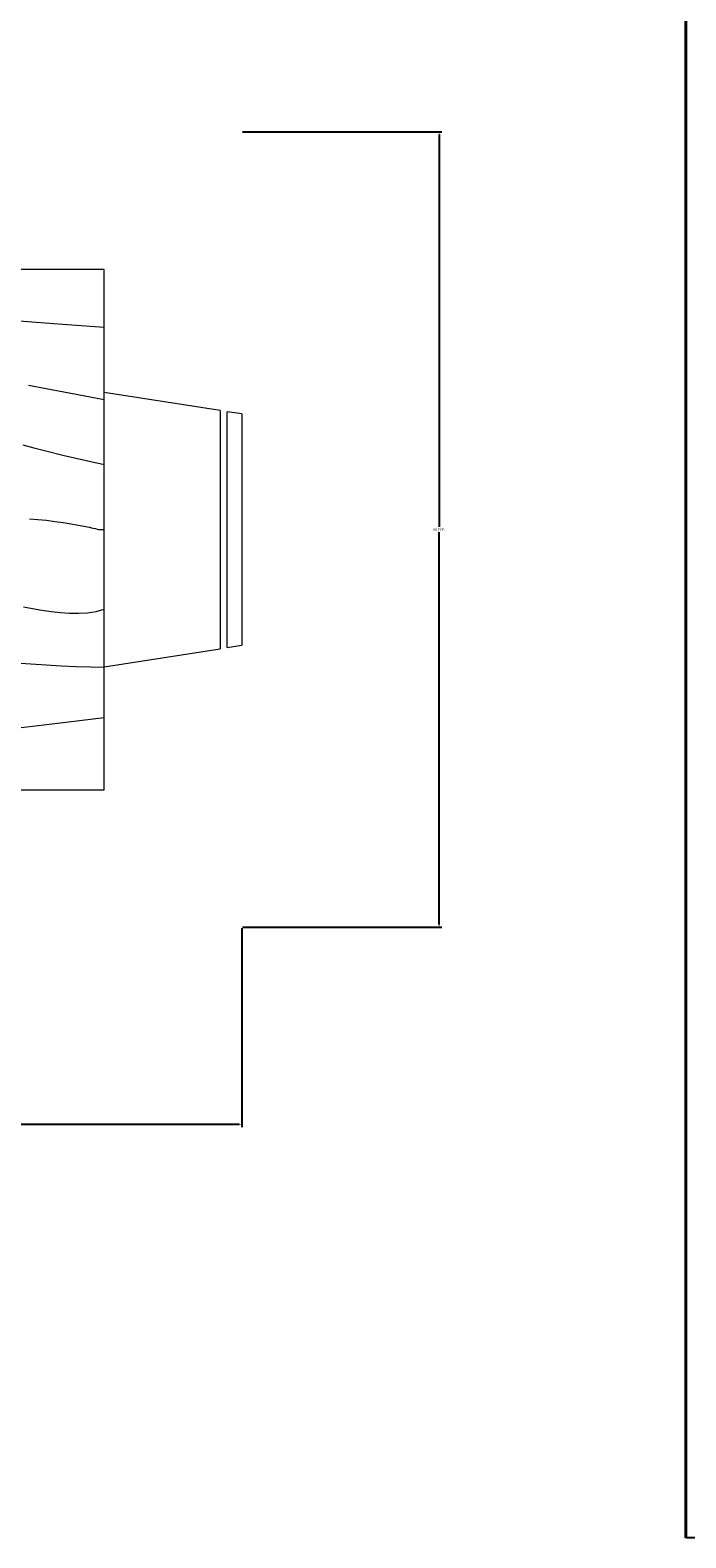
# Model space of a CAD drawing. Units: inches. Extents: x -46 to 1145, y -527 to 760.
# Tile 47 of 57: x 288 to 334, y 367 to 472. Entities that reach past the tile are written whole.
import ezdxf

# ---------------------------------------------------------------- set-up
doc = ezdxf.new("R2010")
doc.units = ezdxf.units.IN
doc.header["$MEASUREMENT"] = 0
for name, color, linetype, lineweight in [('A-ANNO-DIMS', 2, 'Continuous', 18), ('A-FURN', 2, 'Continuous', 13), ('DOORS', 3, 'Continuous', 25), ('WALLS', 4, 'Continuous', 40)]:
    doc.layers.add(name, color=color, linetype=linetype, lineweight=lineweight)
doc.styles.get("Standard").update_dxf_attribs({"font": 'arial.ttf'})
doc.dimstyles.get("Standard").update_dxf_attribs({"dimtxt": 0.18, "dimasz": 0.18, "dimexe": 0.18, "dimexo": 0.0625, "dimgap": 0.09, "dimtad": 0, "dimtih": 1, "dimtoh": 1, "dimdec": 0, "dimzin": 0, "dimdsep": 46, "dimlunit": 3, "dimtxsty": 'Standard', "dimcen": 0.09, "dimadec": 0, "dimazin": 0, "dimtfac": 1, "dimtdec": 0, "dimtofl": 0, "dimtmove": 0, "dimatfit": 3, "dimfxl": 1, "dimtolj": 1, "dimtzin": 0, "dimarcsym": 0})

# ---------------------------------------------------------------- blocks, each defined once
blk = doc.blocks.new('*U2')
for p, q in [((0, 0), (0, -6)), ((40, 0), (40, -6))]:
    blk.add_line(p, q)
blk.add_lwpolyline([(0, 0), (0, 40), (1.75, 40), (1.75, 0)], close=True)
blk.add_arc((0, 0), 40, 0, 90)
blk = doc.blocks.new('Dining Set - 36 x 72 in.')
for p, q in [((36, 18), (-36, 18)), ((36, -18), (36, 18)), ((44.0006, 8.23428), (35.9976, 9.48474)), ((44, 8.23041), (44, -8.23915)), ((44.5, -8.15843), (44.5, 8.15338)), ((45.5, 8), (44.5005, 8.15617)), ((45.5, 8), (45.5, -8)), ((35.9976, -9.48476), (43.9993, -8.2345)), ((44.4997, -8.15631), (45.5, -8)), ((-36, -18), (36, -18))]:
    blk.add_line(p, q)
for points in [[(28.6809, 14.5581), (30.9929, 14.3737), (33.4347, 14.18733), (36, 14)], [(30.752, 9.99414), (33.1936, 9.52856), (36, 9)], [(30.3661, 5.87044), (31.1354, 5.66666), (32.0493, 5.43164), (33.142, 5.16146), (34.4475, 4.85221), (36, 4.5)], [(30.8334, 0.75), (31.4088, 0.70784), (31.9994, 0.64713), (32.589, 0.57275), (33.1615, 0.48958), (33.7008, 0.4025), (34.1908, 0.3164), (34.6153, 0.23616), (34.9584, 0.16666), (35.2099, 0.11165), (35.3848, 0.07031), (35.504, 0.04069), (35.5886, 0.02083), (35.6594, 0.00879), (35.7377, 0.0026), (35.8442, 0.00032), (36, 0)], [(30.4016, -5.34709), (31.0417, -5.45834), (31.6837, -5.56437), (32.3262, -5.65821), (32.9658, -5.73153), (33.599, -5.77604), (34.2224, -5.78345), (34.8327, -5.74545), (35.4264, -5.65373), (36, -5.5)], [(29.8828, -9.20117), (30.93, -9.27824), (31.9792, -9.34896), (33.0205, -9.40991), (34.0443, -9.45768), (35.0407, -9.48885), (36, -9.5)], [(28.2624, -13.9069), (31.8277, -13.50594), (36, -13)]]:
    blk.add_lwpolyline(points)
blk = doc.blocks.new('*D676')
at = {"layer": 'A-ANNO-DIMS', "color": 0, "lineweight": -2, "transparency": 16777216}
for p, q in [((211.86, 409.39), (211.86, 395.63)), ((302.86, 409.39), (302.86, 395.63)), ((212.04, 395.81), (256.08, 395.81)), ((302.68, 395.81), (258.64, 395.81))]:
    blk.add_line(p, q, dxfattribs=at)
at = {"layer": 'A-ANNO-DIMS', "color": 0, "transparency": 16777216}
for points in [[(212.04, 395.84), (212.04, 395.78), (211.86, 395.81)], [(302.68, 395.84), (302.68, 395.78), (302.86, 395.81)]]:
    blk.add_solid(points, dxfattribs=at)
at = {"layer": 'Defpoints', "color": 0, "transparency": 16777216}
for p in [(211.86, 409.46), (302.86, 409.46), (302.86, 395.81)]:
    blk.add_point(p, dxfattribs=at)
at = {"layer": 'A-ANNO-DIMS', "color": 0, "transparency": 16777216, "insert": (257.36, 395.81), "char_height": 0.18, "attachment_point": 5}
blk.add_mtext('\\A1;DINING SET 91 TYP.', dxfattribs=at)
blk = doc.blocks.new('*D677')
at = {"layer": 'A-ANNO-DIMS', "color": 0, "lineweight": -2, "transparency": 16777216}
for p, q in [((302.92, 464.46), (316.69, 464.46)), ((316.51, 464.28), (316.51, 437.14)), ((316.51, 409.64), (316.51, 436.78)), ((302.92, 409.46), (316.69, 409.46))]:
    blk.add_line(p, q, dxfattribs=at)
at = {"layer": 'A-ANNO-DIMS', "color": 0, "transparency": 16777216}
for points in [[(316.48, 464.28), (316.54, 464.28), (316.51, 464.46)], [(316.48, 409.64), (316.54, 409.64), (316.51, 409.46)]]:
    blk.add_solid(points, dxfattribs=at)
at = {"layer": 'Defpoints', "color": 0, "transparency": 16777216}
for p in [(302.86, 464.46), (316.51, 464.46), (302.86, 409.46)]:
    blk.add_point(p, dxfattribs=at)
at = {"layer": 'A-ANNO-DIMS', "color": 0, "transparency": 16777216, "insert": (316.51, 436.96), "char_height": 0.18, "attachment_point": 5}
blk.add_mtext('\\A1;55 TYP.', dxfattribs=at)

msp = doc.modelspace()

# ---------------------------------------------------------------- linework, layer by layer
at = {"layer": 'WALLS'}
msp.add_line((333.5637, 475.5176), (333.5637, 367.232), dxfattribs=at)

# ---------------------------------------------------------------- block references
at = {"layer": 'A-FURN'}
msp.add_blockref('Dining Set - 36 x 72 in.', (257.3617, 436.9572), dxfattribs=at)
at = {"layer": 'DOORS', "xscale": 0.9, "yscale": 0.9, "zscale": 0.9, "rotation": 270}
msp.add_blockref('*U2', (338.9637, 367.232), dxfattribs=at)

# ---------------------------------------------------------------- dimensions: what is measured, and where the dimension line sits
at = {"layer": 'A-ANNO-DIMS'}
dim = msp.add_linear_dim(base=(316.5117, 464.4572), p1=(302.8617, 409.4572), p2=(302.8617, 464.4572), angle=90, text='<> TYP.', dimstyle='Standard', override={"dimdec": 0, "dimlfac": 1, "dimrnd": 0, "dimzin": 0, "dimdsep": 46, "dimlunit": 2}, dxfattribs=at)
dim.commit()
dim.dimension.update_dxf_attribs({"geometry": '*D677', "text_midpoint": (316.5117, 436.9572)})
dim = msp.add_linear_dim(base=(302.8617, 395.8072), p1=(211.8617, 409.4572), p2=(302.8617, 409.4572), text='DINING SET <> TYP.', dimstyle='Standard', override={"dimdec": 0, "dimlfac": 1, "dimrnd": 0, "dimzin": 0, "dimdsep": 46, "dimlunit": 2}, dxfattribs=at)
dim.commit()
dim.dimension.update_dxf_attribs({"geometry": '*D676', "text_midpoint": (257.3617, 395.8072)})

doc.saveas('drawing.dxf')
